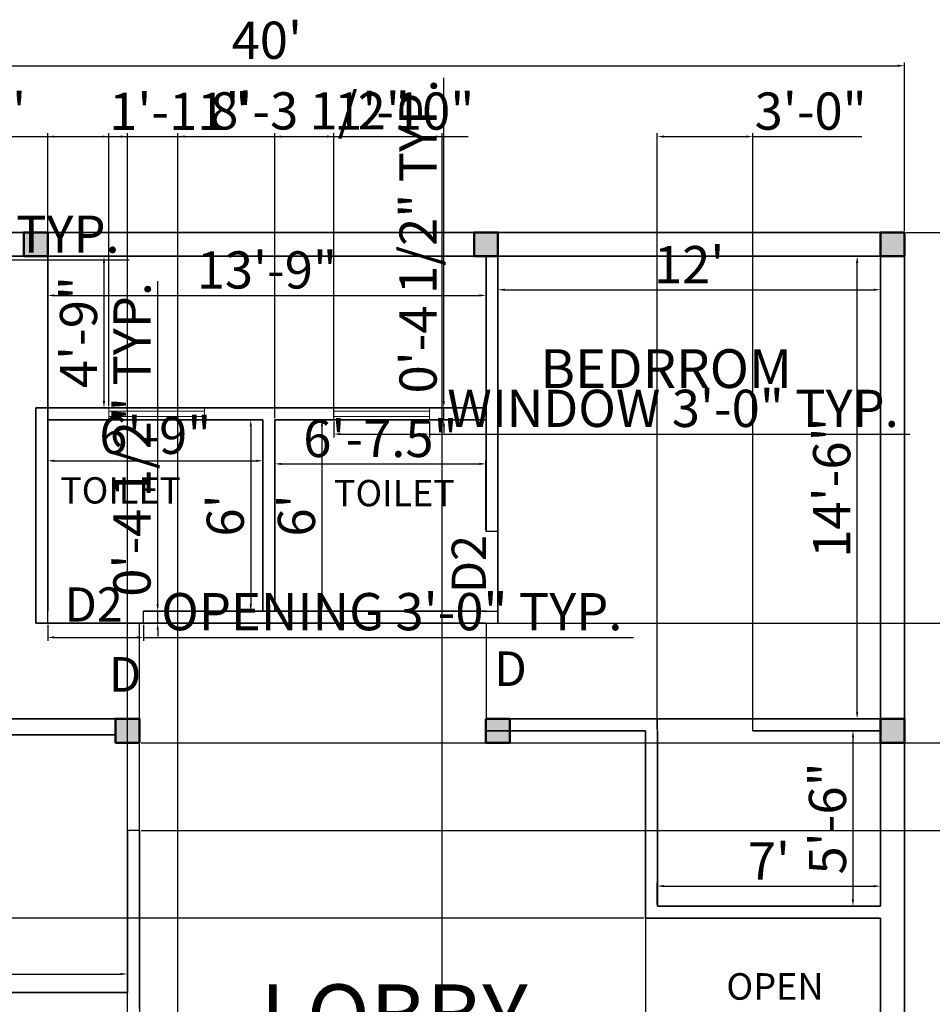
# Model space of a CAD drawing. Units: inches. Extents: x 3316 to 4157, y 2203 to 2977.
# Tile 3 of 4: x 3517 to 3860, y 2597 to 2968. Entities that reach past the tile are written whole.
import ezdxf

# ---------------------------------------------------------------- set-up
doc = ezdxf.new("R2010")
doc.units = ezdxf.units.IN
for name, color, linetype, lineweight in [('A-ANNO-DIMS', 2, 'Continuous', 18), ('A-ANNO-TEXT', 7, 'Continuous', 18), ('A-AREA-IDEN', 7, 'Continuous', 25), ('A-COLS', 7, 'Continuous', 50), ('A-COLS-PATT', 4, 'Continuous', 13), ('A-DOOR', 3, 'Continuous', 25), ('A-GLAZ', 4, 'Continuous', 18), ('A-WALL', 7, 'Continuous', 35), ('C-PROP', 7, 'Continuous', 35)]:
    doc.layers.add(name, color=color, linetype=linetype, lineweight=lineweight)
doc.styles.get("Standard").update_dxf_attribs({"font": 'arial.ttf'})
doc.dimstyles.new('ISO-25', dxfattribs={"dimtxt": 14, "dimasz": 2.5, "dimexe": 1.25, "dimexo": 0.625, "dimtad": 1, "dimlunit": 3, "dimtxsty": 'Standard', "dimcen": 2.5, "dimadec": 0, "dimazin": 0, "dimtfac": 1, "dimtmove": 0, "dimatfit": 3, "dimfxl": 1, "dimarcsym": 0})

# ---------------------------------------------------------------- blocks, each defined once
blk = doc.blocks.new('*D1')
at = {"layer": 'A-ANNO-DIMS', "color": 0, "lineweight": -2, "transparency": 16777216}
for p, q in [((3696.58, 2866.89), (3696.58, 2867.51)), ((3840.58, 2863.07), (3840.58, 2867.51)), ((3699.08, 2866.26), (3838.08, 2866.26))]:
    blk.add_line(p, q, dxfattribs=at)
at = {"layer": 'A-ANNO-DIMS', "color": 0, "transparency": 16777216}
for points in [[(3699.08, 2866.68), (3699.08, 2865.84), (3696.58, 2866.26)], [(3838.08, 2866.68), (3838.08, 2865.84), (3840.58, 2866.26)]]:
    blk.add_solid(points, dxfattribs=at)
at = {"layer": 'Defpoints', "color": 0, "transparency": 16777216}
for p in [(3696.58, 2866.26), (3840.58, 2866.26), (3840.58, 2862.44)]:
    blk.add_point(p, dxfattribs=at)
at = {"layer": 'A-ANNO-DIMS', "color": 0, "transparency": 16777216, "insert": (3768.58, 2873.91), "char_height": 14, "attachment_point": 5}
blk.add_mtext("12'", dxfattribs=at)
blk = doc.blocks.new('*D2')
at = {"layer": 'A-ANNO-DIMS', "color": 0, "lineweight": -2, "transparency": 16777216}
for p, q in [((3832.43, 2878.84), (3833.05, 2878.84)), ((3831.8, 2707.34), (3831.8, 2876.34)), ((3832.43, 2704.84), (3833.05, 2704.84))]:
    blk.add_line(p, q, dxfattribs=at)
at = {"layer": 'A-ANNO-DIMS', "color": 0, "transparency": 16777216}
for points in [[(3831.38, 2876.34), (3832.22, 2876.34), (3831.8, 2878.84)], [(3831.38, 2707.34), (3832.22, 2707.34), (3831.8, 2704.84)]]:
    blk.add_solid(points, dxfattribs=at)
at = {"layer": 'Defpoints', "color": 0, "transparency": 16777216}
for p in [(3831.8, 2878.84), (3831.8, 2878.84), (3831.8, 2704.84)]:
    blk.add_point(p, dxfattribs=at)
at = {"layer": 'A-ANNO-DIMS', "color": 0, "transparency": 16777216, "insert": (3824.03, 2791.84), "char_height": 14, "attachment_point": 5, "rotation": 90}
blk.add_mtext('14\'-6"', dxfattribs=at)
blk = doc.blocks.new('*D6')
at = {"layer": 'A-ANNO-DIMS', "color": 0, "lineweight": -2, "transparency": 16777216}
for p, q in [((3369.58, 2888.47), (3369.58, 2951.81)), ((3372.08, 2950.56), (3847.08, 2950.56)), ((3849.58, 2888.47), (3849.58, 2951.81))]:
    blk.add_line(p, q, dxfattribs=at)
at = {"layer": 'A-ANNO-DIMS', "color": 0, "transparency": 16777216}
for points in [[(3372.08, 2950.98), (3372.08, 2950.14), (3369.58, 2950.56)], [(3847.08, 2950.98), (3847.08, 2950.14), (3849.58, 2950.56)]]:
    blk.add_solid(points, dxfattribs=at)
at = {"layer": 'Defpoints', "color": 0, "transparency": 16777216}
for p in [(3849.58, 2950.56), (3369.58, 2887.84), (3849.58, 2887.84)]:
    blk.add_point(p, dxfattribs=at)
at = {"layer": 'A-ANNO-DIMS', "color": 0, "transparency": 16777216, "insert": (3609.58, 2958.33), "char_height": 14, "attachment_point": 5}
blk.add_mtext("40'", dxfattribs=at)
blk = doc.blocks.new('*D7')
at = {"layer": 'A-ANNO-DIMS', "color": 0, "lineweight": -2, "transparency": 16777216}
for p, q in [((3850.21, 2887.84), (4040.36, 2887.84)), ((4039.11, 2885.34), (4039.11, 2254.34)), ((3850.21, 2251.84), (4040.36, 2251.84))]:
    blk.add_line(p, q, dxfattribs=at)
at = {"layer": 'A-ANNO-DIMS', "color": 0, "transparency": 16777216}
for points in [[(4038.69, 2885.34), (4039.53, 2885.34), (4039.11, 2887.84)], [(4038.69, 2254.34), (4039.53, 2254.34), (4039.11, 2251.84)]]:
    blk.add_solid(points, dxfattribs=at)
at = {"layer": 'Defpoints', "color": 0, "transparency": 16777216}
for p in [(3849.58, 2887.84), (3849.58, 2251.84), (4039.11, 2251.84)]:
    blk.add_point(p, dxfattribs=at)
at = {"layer": 'A-ANNO-DIMS', "color": 0, "transparency": 16777216, "insert": (4031.33, 2569.84), "char_height": 14, "attachment_point": 5, "rotation": 90}
blk.add_mtext("53'", dxfattribs=at)
blk = doc.blocks.new('*D8')
at = {"layer": 'A-ANNO-DIMS', "color": 0, "lineweight": -2, "transparency": 16777216}
for p, q in [((3527.08, 2802.53), (3527.08, 2803.15)), ((3529.58, 2801.9), (3605.58, 2801.9)), ((3608.08, 2802.53), (3608.08, 2803.15))]:
    blk.add_line(p, q, dxfattribs=at)
at = {"layer": 'A-ANNO-DIMS', "color": 0, "transparency": 16777216}
for points in [[(3529.58, 2802.32), (3529.58, 2801.48), (3527.08, 2801.9)], [(3605.58, 2802.32), (3605.58, 2801.48), (3608.08, 2801.9)]]:
    blk.add_solid(points, dxfattribs=at)
at = {"layer": 'Defpoints', "color": 0, "transparency": 16777216}
for p in [(3527.08, 2801.9), (3608.08, 2801.9), (3608.08, 2801.9)]:
    blk.add_point(p, dxfattribs=at)
at = {"layer": 'A-ANNO-DIMS', "color": 0, "transparency": 16777216, "insert": (3567.58, 2809.67), "char_height": 14, "attachment_point": 5}
blk.add_mtext('6\'-9"', dxfattribs=at)
blk = doc.blocks.new('*D9')
at = {"layer": 'A-ANNO-DIMS', "color": 0, "lineweight": -2, "transparency": 16777216}
for p, q in [((3613.21, 2817.34), (3631.55, 2817.34)), ((3630.3, 2814.84), (3630.3, 2747.84)), ((3613.21, 2745.34), (3631.55, 2745.34))]:
    blk.add_line(p, q, dxfattribs=at)
at = {"layer": 'A-ANNO-DIMS', "color": 0, "transparency": 16777216}
for points in [[(3629.89, 2814.84), (3630.72, 2814.84), (3630.3, 2817.34)], [(3629.89, 2747.84), (3630.72, 2747.84), (3630.3, 2745.34)]]:
    blk.add_solid(points, dxfattribs=at)
at = {"layer": 'Defpoints', "color": 0, "transparency": 16777216}
for p in [(3612.58, 2817.34), (3612.58, 2745.34), (3630.3, 2745.34)]:
    blk.add_point(p, dxfattribs=at)
at = {"layer": 'A-ANNO-DIMS', "color": 0, "transparency": 16777216, "insert": (3622.53, 2781.34), "char_height": 14, "attachment_point": 5, "rotation": 90}
blk.add_mtext("6'", dxfattribs=at)
blk = doc.blocks.new('*D10')
at = {"layer": 'A-ANNO-DIMS', "color": 0, "lineweight": -2, "transparency": 16777216}
for p, q in [((3612.58, 2816.72), (3612.58, 2799.49)), ((3692.08, 2775.97), (3692.08, 2801.99)), ((3615.08, 2800.74), (3689.58, 2800.74))]:
    blk.add_line(p, q, dxfattribs=at)
at = {"layer": 'A-ANNO-DIMS', "color": 0, "transparency": 16777216}
for points in [[(3615.08, 2801.15), (3615.08, 2800.32), (3612.58, 2800.74)], [(3689.58, 2801.15), (3689.58, 2800.32), (3692.08, 2800.74)]]:
    blk.add_solid(points, dxfattribs=at)
at = {"layer": 'Defpoints', "color": 0, "transparency": 16777216}
for p in [(3612.58, 2817.34), (3692.08, 2800.74), (3692.08, 2775.34)]:
    blk.add_point(p, dxfattribs=at)
at = {"layer": 'A-ANNO-DIMS', "color": 0, "transparency": 16777216, "insert": (3652.33, 2808.51), "char_height": 14, "attachment_point": 5}
blk.add_mtext('6\'-7.5"', dxfattribs=at)
blk = doc.blocks.new('*D15')
at = {"layer": 'A-ANNO-DIMS', "color": 0, "lineweight": -2, "transparency": 16777216}
for p, q in [((3437.08, 2602.47), (3437.08, 2610.05)), ((3439.58, 2608.8), (3554.58, 2608.8)), ((3557.08, 2602.47), (3557.08, 2610.05))]:
    blk.add_line(p, q, dxfattribs=at)
at = {"layer": 'A-ANNO-DIMS', "color": 0, "transparency": 16777216}
for points in [[(3439.58, 2609.21), (3439.58, 2608.38), (3437.08, 2608.8)], [(3554.58, 2609.21), (3554.58, 2608.38), (3557.08, 2608.8)]]:
    blk.add_solid(points, dxfattribs=at)
at = {"layer": 'Defpoints', "color": 0, "transparency": 16777216}
for p in [(3557.08, 2608.8), (3437.08, 2601.84), (3557.08, 2601.84)]:
    blk.add_point(p, dxfattribs=at)
at = {"layer": 'A-ANNO-DIMS', "color": 0, "transparency": 16777216, "insert": (3497.08, 2616.57), "char_height": 14, "attachment_point": 5}
blk.add_mtext("10'", dxfattribs=at)
blk = doc.blocks.new('*D16')
at = {"layer": 'A-ANNO-DIMS', "color": 0, "lineweight": -2, "transparency": 16777216}
for p, q in [((3839.96, 2700.34), (3828.97, 2700.34)), ((3830.22, 2697.84), (3830.22, 2636.84)), ((3839.96, 2634.34), (3828.97, 2634.34))]:
    blk.add_line(p, q, dxfattribs=at)
at = {"layer": 'A-ANNO-DIMS', "color": 0, "transparency": 16777216}
for points in [[(3829.8, 2697.84), (3830.63, 2697.84), (3830.22, 2700.34)], [(3829.8, 2636.84), (3830.63, 2636.84), (3830.22, 2634.34)]]:
    blk.add_solid(points, dxfattribs=at)
at = {"layer": 'Defpoints', "color": 0, "transparency": 16777216}
for p in [(3840.58, 2700.34), (3830.22, 2634.34), (3840.58, 2634.34)]:
    blk.add_point(p, dxfattribs=at)
at = {"layer": 'A-ANNO-DIMS', "color": 0, "transparency": 16777216, "insert": (3822.44, 2667.34), "char_height": 14, "attachment_point": 5, "rotation": 90}
blk.add_mtext('5\'-6"', dxfattribs=at)
blk = doc.blocks.new('*D17')
at = {"layer": 'A-ANNO-DIMS', "color": 0, "lineweight": -2, "transparency": 16777216}
for p, q in [((3756.58, 2634.97), (3756.58, 2643.11)), ((3759.08, 2641.86), (3838.08, 2641.86)), ((3840.58, 2634.97), (3840.58, 2643.11))]:
    blk.add_line(p, q, dxfattribs=at)
at = {"layer": 'A-ANNO-DIMS', "color": 0, "transparency": 16777216}
for points in [[(3759.08, 2642.28), (3759.08, 2641.45), (3756.58, 2641.86)], [(3838.08, 2642.28), (3838.08, 2641.45), (3840.58, 2641.86)]]:
    blk.add_solid(points, dxfattribs=at)
at = {"layer": 'Defpoints', "color": 0, "transparency": 16777216}
for p in [(3840.58, 2641.86), (3756.58, 2634.34), (3840.58, 2634.34)]:
    blk.add_point(p, dxfattribs=at)
at = {"layer": 'A-ANNO-DIMS', "color": 0, "transparency": 16777216, "insert": (3798.58, 2649.49), "char_height": 14, "attachment_point": 5}
blk.add_mtext("7'", dxfattribs=at)
blk = doc.blocks.new('*D22')
at = {"layer": 'A-ANNO-DIMS', "color": 0, "lineweight": -2, "transparency": 16777216}
for p, q in [((3527.08, 2878.22), (3527.08, 2862.87)), ((3692.08, 2878.22), (3692.08, 2862.87)), ((3529.58, 2864.12), (3689.58, 2864.12))]:
    blk.add_line(p, q, dxfattribs=at)
at = {"layer": 'A-ANNO-DIMS', "color": 0, "transparency": 16777216}
for points in [[(3529.58, 2864.54), (3529.58, 2863.7), (3527.08, 2864.12)], [(3689.58, 2864.54), (3689.58, 2863.7), (3692.08, 2864.12)]]:
    blk.add_solid(points, dxfattribs=at)
at = {"layer": 'Defpoints', "color": 0, "transparency": 16777216}
for p in [(3527.08, 2878.84), (3692.08, 2878.84), (3692.08, 2864.12)]:
    blk.add_point(p, dxfattribs=at)
at = {"layer": 'A-ANNO-DIMS', "color": 0, "transparency": 16777216, "insert": (3609.58, 2871.9), "char_height": 14, "attachment_point": 5}
blk.add_mtext('13\'-9"', dxfattribs=at)
blk = doc.blocks.new('*D23')
at = {"layer": 'A-ANNO-DIMS', "color": 0, "lineweight": -2, "transparency": 16777216}
for p, q in [((3527.71, 2878.84), (3549.52, 2878.84)), ((3548.27, 2876.34), (3548.27, 2824.34)), ((3527.71, 2821.84), (3549.52, 2821.84))]:
    blk.add_line(p, q, dxfattribs=at)
at = {"layer": 'A-ANNO-DIMS', "color": 0, "transparency": 16777216}
for points in [[(3547.85, 2876.34), (3548.69, 2876.34), (3548.27, 2878.84)], [(3547.85, 2824.34), (3548.69, 2824.34), (3548.27, 2821.84)]]:
    blk.add_solid(points, dxfattribs=at)
at = {"layer": 'Defpoints', "color": 0, "transparency": 16777216}
for p in [(3527.08, 2878.84), (3527.08, 2821.84), (3548.27, 2821.84)]:
    blk.add_point(p, dxfattribs=at)
at = {"layer": 'A-ANNO-DIMS', "color": 0, "transparency": 16777216, "insert": (3540.5, 2850.34), "char_height": 14, "attachment_point": 5, "rotation": 90}
blk.add_mtext('4\'-9"', dxfattribs=at)
blk = doc.blocks.new('*D26')
at = {"layer": 'A-ANNO-DIMS', "color": 0, "lineweight": -2, "transparency": 16777216}
for p, q in [((3607.46, 2817.34), (3602.26, 2817.34)), ((3603.51, 2814.84), (3603.51, 2747.84)), ((3607.46, 2745.34), (3602.26, 2745.34))]:
    blk.add_line(p, q, dxfattribs=at)
at = {"layer": 'A-ANNO-DIMS', "color": 0, "transparency": 16777216}
for points in [[(3603.1, 2814.84), (3603.93, 2814.84), (3603.51, 2817.34)], [(3603.1, 2747.84), (3603.93, 2747.84), (3603.51, 2745.34)]]:
    blk.add_solid(points, dxfattribs=at)
at = {"layer": 'Defpoints', "color": 0, "transparency": 16777216}
for p in [(3608.08, 2817.34), (3603.51, 2745.34), (3608.08, 2745.34)]:
    blk.add_point(p, dxfattribs=at)
at = {"layer": 'A-ANNO-DIMS', "color": 0, "transparency": 16777216, "insert": (3595.74, 2781.34), "char_height": 14, "attachment_point": 5, "rotation": 90}
blk.add_mtext("6'", dxfattribs=at)
blk = doc.blocks.new('COL-9IN-SQ')
for p, q in [((0, 9), (0, 0)), ((9, 9), (0, 9)), ((9, 0), (9, 9)), ((0, 0), (9, 0))]:
    blk.add_line(p, q)
blk = doc.blocks.new('COL-9IN-SQ-PL')
blk.add_lwpolyline([(0, 0), (9, 0), (9, 9), (0, 9)], close=True)
blk = doc.blocks.new('WIN-36IN')
for p, q in [((0, 0), (0, 4.5)), ((36, 4.5), (36, 0)), ((0, 3.25), (36, 3.25)), ((0, 1.25), (36, 1.25)), ((36, 0), (0, 0))]:
    blk.add_line(p, q)
blk = doc.blocks.new('DOOR-36IN-OPENING')
for p, q in [((0, 0), (0, 4.5)), ((36, 0), (36, 4.5)), ((0, 0), (36, 0))]:
    blk.add_line(p, q)
blk = doc.blocks.new('DOOR-30IN-OPENING')
for p, q in [((4.5, 30), (0, 30)), ((4.5, 0), (4.5, 30)), ((0, 0), (4.5, 0))]:
    blk.add_line(p, q)
blk = doc.blocks.new('*D36')
at = {"layer": 'A-ANNO-DIMS', "color": 0, "lineweight": -2, "transparency": 16777216}
for p, q in [((3369.58, 2878.22), (3369.58, 2876.24)), ((3372.08, 2877.49), (3376.08, 2877.49)), ((3378.58, 2878.22), (3378.58, 2876.24)), ((3378.58, 2877.49), (3557.7, 2877.49))]:
    blk.add_line(p, q, dxfattribs=at)
at = {"layer": 'A-ANNO-DIMS', "color": 0, "transparency": 16777216}
for points in [[(3372.08, 2877.91), (3372.08, 2877.08), (3369.58, 2877.49)], [(3376.08, 2877.91), (3376.08, 2877.08), (3378.58, 2877.49)]]:
    blk.add_solid(points, dxfattribs=at)
at = {"layer": 'Defpoints', "color": 0, "transparency": 16777216}
for p in [(3369.58, 2878.84), (3378.58, 2878.84), (3378.58, 2877.49)]:
    blk.add_point(p, dxfattribs=at)
at = {"layer": 'A-ANNO-DIMS', "color": 0, "transparency": 16777216, "insert": (3469.39, 2885.36), "char_height": 14, "attachment_point": 5}
blk.add_mtext('COLUMN 0\'-9" TYP.', dxfattribs=at)
blk = doc.blocks.new('*D40')
at = {"layer": 'A-ANNO-DIMS', "color": 0, "lineweight": -2, "transparency": 16777216}
for p, q in [((3634.78, 2816.72), (3634.78, 2810.69)), ((3670.78, 2816.72), (3670.78, 2810.69)), ((3637.28, 2811.94), (3668.28, 2811.94)), ((3670.78, 2811.94), (3851.69, 2811.94))]:
    blk.add_line(p, q, dxfattribs=at)
at = {"layer": 'A-ANNO-DIMS', "color": 0, "transparency": 16777216}
for points in [[(3637.28, 2812.36), (3637.28, 2811.53), (3634.78, 2811.94)], [(3668.28, 2812.36), (3668.28, 2811.53), (3670.78, 2811.94)]]:
    blk.add_solid(points, dxfattribs=at)
at = {"layer": 'Defpoints', "color": 0, "transparency": 16777216}
for p in [(3634.78, 2817.34), (3670.78, 2817.34), (3670.78, 2811.94)]:
    blk.add_point(p, dxfattribs=at)
at = {"layer": 'A-ANNO-DIMS', "color": 0, "transparency": 16777216, "insert": (3762.48, 2819.82), "char_height": 14, "attachment_point": 5}
blk.add_mtext('WINDOW 3\'-0" TYP.', dxfattribs=at)
blk = doc.blocks.new('*D41')
at = {"layer": 'A-ANNO-DIMS', "color": 0, "lineweight": -2, "transparency": 16777216}
for p, q in [((3676.18, 2824.34), (3676.18, 2946.05)), ((3671.41, 2821.84), (3677.43, 2821.84)), ((3676.18, 2817.34), (3676.18, 2821.84)), ((3671.41, 2817.34), (3677.43, 2817.34)), ((3676.18, 2814.84), (3676.18, 2812.34))]:
    blk.add_line(p, q, dxfattribs=at)
at = {"layer": 'A-ANNO-DIMS', "color": 0, "transparency": 16777216}
for points in [[(3675.76, 2824.34), (3676.6, 2824.34), (3676.18, 2821.84)], [(3675.76, 2814.84), (3676.6, 2814.84), (3676.18, 2817.34)]]:
    blk.add_solid(points, dxfattribs=at)
at = {"layer": 'Defpoints', "color": 0, "transparency": 16777216}
for p in [(3670.78, 2821.84), (3676.18, 2821.84), (3670.78, 2817.34)]:
    blk.add_point(p, dxfattribs=at)
at = {"layer": 'A-ANNO-DIMS', "color": 0, "transparency": 16777216, "insert": (3668.32, 2886.45), "char_height": 14, "attachment_point": 5, "rotation": 90}
blk.add_mtext('0\'-4 1/2" TYP.', dxfattribs=at)
blk = doc.blocks.new('*D42')
at = {"layer": 'A-ANNO-DIMS', "color": 0, "lineweight": -2, "transparency": 16777216}
for p, q in [((3527.08, 2740.22), (3527.08, 2734.19)), ((3563.08, 2740.22), (3563.08, 2734.19)), ((3529.58, 2735.44), (3560.58, 2735.44)), ((3563.08, 2735.44), (3747.67, 2735.44))]:
    blk.add_line(p, q, dxfattribs=at)
at = {"layer": 'A-ANNO-DIMS', "color": 0, "transparency": 16777216}
for points in [[(3529.58, 2735.86), (3529.58, 2735.03), (3527.08, 2735.44)], [(3560.58, 2735.86), (3560.58, 2735.03), (3563.08, 2735.44)]]:
    blk.add_solid(points, dxfattribs=at)
at = {"layer": 'Defpoints', "color": 0, "transparency": 16777216}
for p in [(3527.08, 2740.84), (3563.08, 2740.84), (3563.08, 2735.44)]:
    blk.add_point(p, dxfattribs=at)
at = {"layer": 'A-ANNO-DIMS', "color": 0, "transparency": 16777216, "insert": (3656.63, 2743.32), "char_height": 14, "attachment_point": 5}
blk.add_mtext('OPENING 3\'-0" TYP.', dxfattribs=at)
blk = doc.blocks.new('*D43')
at = {"layer": 'A-ANNO-DIMS', "color": 0, "lineweight": -2, "transparency": 16777216}
for p, q in [((3568.48, 2747.84), (3568.48, 2869.55)), ((3563.71, 2745.34), (3569.73, 2745.34)), ((3568.48, 2740.84), (3568.48, 2745.34)), ((3563.71, 2740.84), (3569.73, 2740.84)), ((3568.48, 2738.34), (3568.48, 2735.84))]:
    blk.add_line(p, q, dxfattribs=at)
at = {"layer": 'A-ANNO-DIMS', "color": 0, "transparency": 16777216}
for points in [[(3568.07, 2747.84), (3568.9, 2747.84), (3568.48, 2745.34)], [(3568.07, 2738.34), (3568.9, 2738.34), (3568.48, 2740.84)]]:
    blk.add_solid(points, dxfattribs=at)
at = {"layer": 'Defpoints', "color": 0, "transparency": 16777216}
for p in [(3563.08, 2745.34), (3568.48, 2745.34), (3563.08, 2740.84)]:
    blk.add_point(p, dxfattribs=at)
at = {"layer": 'A-ANNO-DIMS', "color": 0, "transparency": 16777216, "insert": (3560.62, 2809.95), "char_height": 14, "attachment_point": 5, "rotation": 90}
blk.add_mtext('0\'-4 1/2" TYP.', dxfattribs=at)
blk = doc.blocks.new('*D48')
at = {"layer": 'A-ANNO-DIMS', "color": 0, "lineweight": -2, "transparency": 16777216}
for p, q in [((3527.08, 2822.47), (3527.08, 2925.14)), ((3529.58, 2923.89), (3547.61, 2923.89)), ((3550.11, 2822.47), (3550.11, 2925.14)), ((3550.11, 2923.89), (3600.63, 2923.89))]:
    blk.add_line(p, q, dxfattribs=at)
at = {"layer": 'A-ANNO-DIMS', "color": 0, "transparency": 16777216}
for points in [[(3529.58, 2924.31), (3529.58, 2923.48), (3527.08, 2923.89)], [(3547.61, 2924.31), (3547.61, 2923.48), (3550.11, 2923.89)]]:
    blk.add_solid(points, dxfattribs=at)
at = {"layer": 'Defpoints', "color": 0, "transparency": 16777216}
for p in [(3550.11, 2923.89), (3527.08, 2821.84), (3550.11, 2821.84)]:
    blk.add_point(p, dxfattribs=at)
at = {"layer": 'A-ANNO-DIMS', "color": 0, "transparency": 16777216, "insert": (3576.62, 2931.55), "char_height": 14, "attachment_point": 5}
blk.add_mtext('1\'-11"', dxfattribs=at)
blk = doc.blocks.new('*D49')
at = {"layer": 'A-ANNO-DIMS', "color": 0, "lineweight": -2, "transparency": 16777216}
for p, q in [((3612.58, 2817.97), (3612.58, 2925.14)), ((3615.08, 2923.89), (3632.28, 2923.89)), ((3634.78, 2817.97), (3634.78, 2925.14)), ((3634.78, 2923.89), (3685.31, 2923.89))]:
    blk.add_line(p, q, dxfattribs=at)
at = {"layer": 'A-ANNO-DIMS', "color": 0, "transparency": 16777216}
for points in [[(3615.08, 2924.31), (3615.08, 2923.48), (3612.58, 2923.89)], [(3632.28, 2924.31), (3632.28, 2923.48), (3634.78, 2923.89)]]:
    blk.add_solid(points, dxfattribs=at)
at = {"layer": 'Defpoints', "color": 0, "transparency": 16777216}
for p in [(3634.78, 2923.89), (3612.58, 2817.34), (3634.78, 2817.34)]:
    blk.add_point(p, dxfattribs=at)
at = {"layer": 'A-ANNO-DIMS', "color": 0, "transparency": 16777216, "insert": (3661.29, 2931.67), "char_height": 14, "attachment_point": 5}
blk.add_mtext('1\'-10"', dxfattribs=at)
blk = doc.blocks.new('*D50')
at = {"layer": 'A-ANNO-DIMS', "color": 0, "lineweight": -2, "transparency": 16777216}
for p, q in [((3751.46, 2629.84), (3332.28, 2629.84)), ((3333.53, 2627.34), (3333.53, 2578.34)), ((3751.46, 2575.84), (3332.28, 2575.84))]:
    blk.add_line(p, q, dxfattribs=at)
at = {"layer": 'A-ANNO-DIMS', "color": 0, "transparency": 16777216}
for points in [[(3333.12, 2627.34), (3333.95, 2627.34), (3333.53, 2629.84)], [(3333.12, 2578.34), (3333.95, 2578.34), (3333.53, 2575.84)]]:
    blk.add_solid(points, dxfattribs=at)
at = {"layer": 'Defpoints', "color": 0, "transparency": 16777216}
for p in [(3752.08, 2629.84), (3333.53, 2575.84), (3752.08, 2575.84)]:
    blk.add_point(p, dxfattribs=at)
at = {"layer": 'A-ANNO-DIMS', "color": 0, "transparency": 16777216, "insert": (3325.76, 2602.84), "char_height": 14, "attachment_point": 5, "rotation": 90}
blk.add_mtext('4\'-6"', dxfattribs=at)
blk = doc.blocks.new('*D51')
at = {"layer": 'A-ANNO-DIMS', "color": 0, "lineweight": -2, "transparency": 16777216}
for p, q in [((3562.21, 2695.84), (3886.88, 2695.84)), ((3885.63, 2693.34), (3885.63, 2665.34)), ((3562.21, 2662.84), (3886.88, 2662.84)), ((3885.63, 2662.84), (3885.63, 2621.64))]:
    blk.add_line(p, q, dxfattribs=at)
at = {"layer": 'A-ANNO-DIMS', "color": 0, "transparency": 16777216}
for points in [[(3885.22, 2693.34), (3886.05, 2693.34), (3885.63, 2695.84)], [(3885.22, 2665.34), (3886.05, 2665.34), (3885.63, 2662.84)]]:
    blk.add_solid(points, dxfattribs=at)
at = {"layer": 'Defpoints', "color": 0, "transparency": 16777216}
for p in [(3561.58, 2695.84), (3561.58, 2662.84), (3885.63, 2662.84)]:
    blk.add_point(p, dxfattribs=at)
at = {"layer": 'A-ANNO-DIMS', "color": 0, "transparency": 16777216, "insert": (3877.86, 2640.99), "char_height": 14, "attachment_point": 5, "rotation": 90}
blk.add_mtext('2\'-9"', dxfattribs=at)
blk = doc.blocks.new('*D52')
at = {"layer": 'A-ANNO-DIMS', "color": 0, "lineweight": -2, "transparency": 16777216}
for p, q in [((3576.12, 2505.97), (3576.12, 2925.14)), ((3578.62, 2923.89), (3673.07, 2923.89)), ((3675.57, 2505.97), (3675.57, 2925.14))]:
    blk.add_line(p, q, dxfattribs=at)
at = {"layer": 'A-ANNO-DIMS', "color": 0, "transparency": 16777216}
for points in [[(3578.62, 2924.31), (3578.62, 2923.48), (3576.12, 2923.89)], [(3673.07, 2924.31), (3673.07, 2923.48), (3675.57, 2923.89)]]:
    blk.add_solid(points, dxfattribs=at)
at = {"layer": 'Defpoints', "color": 0, "transparency": 16777216}
for p in [(3675.57, 2923.89), (3576.12, 2505.34), (3675.57, 2505.34)]:
    blk.add_point(p, dxfattribs=at)
at = {"layer": 'A-ANNO-DIMS', "color": 0, "transparency": 16777216, "insert": (3625.84, 2931.76), "char_height": 14, "attachment_point": 5}
blk.add_mtext('8\'-3 1/2"', dxfattribs=at)
blk = doc.blocks.new('*D56')
at = {"layer": 'A-ANNO-DIMS', "color": 0, "lineweight": -2, "transparency": 16777216}
for p, q in [((3752.08, 2699.72), (3752.08, 2214.54)), ((3561.58, 2662.22), (3561.58, 2214.54)), ((3564.08, 2215.79), (3749.58, 2215.79))]:
    blk.add_line(p, q, dxfattribs=at)
at = {"layer": 'A-ANNO-DIMS', "color": 0, "transparency": 16777216}
for points in [[(3564.08, 2216.21), (3564.08, 2215.38), (3561.58, 2215.79)], [(3749.58, 2216.21), (3749.58, 2215.38), (3752.08, 2215.79)]]:
    blk.add_solid(points, dxfattribs=at)
at = {"layer": 'Defpoints', "color": 0, "transparency": 16777216}
for p in [(3752.08, 2700.34), (3561.58, 2662.84), (3752.08, 2215.79)]:
    blk.add_point(p, dxfattribs=at)
at = {"layer": 'A-ANNO-DIMS', "color": 0, "transparency": 16777216, "insert": (3656.83, 2223.66), "char_height": 14, "attachment_point": 5}
blk.add_mtext('15\'-10 1/2"', dxfattribs=at)
blk = doc.blocks.new('*D57')
at = {"layer": 'A-ANNO-DIMS', "color": 0, "lineweight": -2, "transparency": 16777216}
for p, q in [((3692.71, 2740.84), (3886.88, 2740.84)), ((3885.63, 2507.84), (3885.63, 2738.34)), ((3676.19, 2505.34), (3886.88, 2505.34))]:
    blk.add_line(p, q, dxfattribs=at)
at = {"layer": 'A-ANNO-DIMS', "color": 0, "transparency": 16777216}
for points in [[(3885.22, 2738.34), (3886.05, 2738.34), (3885.63, 2740.84)], [(3885.22, 2507.84), (3886.05, 2507.84), (3885.63, 2505.34)]]:
    blk.add_solid(points, dxfattribs=at)
at = {"layer": 'Defpoints', "color": 0, "transparency": 16777216}
for p in [(3692.08, 2740.84), (3885.63, 2740.84), (3675.57, 2505.34)]:
    blk.add_point(p, dxfattribs=at)
at = {"layer": 'A-ANNO-DIMS', "color": 0, "transparency": 16777216, "insert": (3877.77, 2623.09), "char_height": 14, "attachment_point": 5, "rotation": 90}
blk.add_mtext('19\'-7 1/2"', dxfattribs=at)
blk = doc.blocks.new('*D58')
at = {"layer": 'A-ANNO-DIMS', "color": 0, "lineweight": -2, "transparency": 16777216}
for p, q in [((3756.58, 2700.97), (3756.58, 2925.14)), ((3759.08, 2923.89), (3790.08, 2923.89)), ((3792.58, 2700.97), (3792.58, 2925.14)), ((3792.58, 2923.89), (3833.54, 2923.89))]:
    blk.add_line(p, q, dxfattribs=at)
at = {"layer": 'A-ANNO-DIMS', "color": 0, "transparency": 16777216}
for points in [[(3759.08, 2924.31), (3759.08, 2923.48), (3756.58, 2923.89)], [(3790.08, 2924.31), (3790.08, 2923.48), (3792.58, 2923.89)]]:
    blk.add_solid(points, dxfattribs=at)
at = {"layer": 'Defpoints', "color": 0, "transparency": 16777216}
for p in [(3792.58, 2923.89), (3756.58, 2700.34), (3792.58, 2700.34)]:
    blk.add_point(p, dxfattribs=at)
at = {"layer": 'A-ANNO-DIMS', "color": 0, "transparency": 16777216, "insert": (3814.31, 2931.67), "char_height": 14, "attachment_point": 5}
blk.add_mtext('3\'-0"', dxfattribs=at)
blk = doc.blocks.new('*D60')
at = {"layer": 'A-ANNO-DIMS', "color": 0, "lineweight": -2, "transparency": 16777216}
for p, q in [((3428.08, 2544.97), (3428.08, 2925.14)), ((3430.58, 2923.89), (3554.58, 2923.89)), ((3557.08, 2544.97), (3557.08, 2925.14))]:
    blk.add_line(p, q, dxfattribs=at)
at = {"layer": 'A-ANNO-DIMS', "color": 0, "transparency": 16777216}
for points in [[(3430.58, 2924.31), (3430.58, 2923.48), (3428.08, 2923.89)], [(3554.58, 2924.31), (3554.58, 2923.48), (3557.08, 2923.89)]]:
    blk.add_solid(points, dxfattribs=at)
at = {"layer": 'Defpoints', "color": 0, "transparency": 16777216}
for p in [(3557.08, 2923.89), (3428.08, 2544.34), (3557.08, 2544.34)]:
    blk.add_point(p, dxfattribs=at)
at = {"layer": 'A-ANNO-DIMS', "color": 0, "transparency": 16777216, "insert": (3492.58, 2931.67), "char_height": 14, "attachment_point": 5}
blk.add_mtext('10\'-9"', dxfattribs=at)

msp = doc.modelspace()

# ---------------------------------------------------------------- hatches: boundary and pattern name
at = {"layer": 'A-COLS-PATT'}
h = msp.add_hatch(color=256, dxfattribs=at)
h.dxf.hatch_style = 1
h.paths.add_polyline_path([(3849.584, 2887.842), (3840.584, 2887.842), (3840.584, 2878.842), (3849.584, 2878.842)])
h.paths.add_polyline_path([(3696.584, 2887.842), (3687.584, 2887.842), (3687.584, 2878.842), (3696.584, 2878.842)])
h.paths.add_polyline_path([(3527.084, 2887.842), (3518.084, 2887.842), (3518.084, 2878.842), (3527.084, 2878.842)])
h.paths.add_polyline_path([(3378.584, 2887.842), (3369.584, 2887.842), (3369.584, 2878.842), (3378.584, 2878.842)])
h.paths.add_polyline_path([(3378.584, 2707.842), (3369.584, 2707.842), (3369.584, 2698.842), (3378.584, 2698.842)])
h.paths.add_polyline_path([(3561.584, 2704.842), (3552.584, 2704.842), (3552.584, 2695.842), (3561.584, 2695.842)])
h.paths.add_polyline_path([(3701.03, 2704.842), (3692.084, 2704.842), (3692.084, 2700.342), (3701.03, 2700.342)])
h.paths.add_polyline_path([(3701.03, 2700.342), (3692.03, 2700.342), (3692.03, 2695.842), (3701.03, 2695.842)])
h.paths.add_polyline_path([(3849.584, 2704.835), (3840.584, 2704.835), (3840.584, 2695.835), (3849.584, 2695.835)])
h.paths.add_polyline_path([(3378.584, 2505.342), (3369.584, 2505.342), (3369.584, 2496.342), (3378.584, 2496.342)])
h.paths.add_polyline_path([(3378.584, 2357.104), (3369.584, 2357.104), (3369.584, 2348.104), (3378.584, 2348.104)])
h.paths.add_polyline_path([(3512.084, 2505.342), (3503.084, 2505.342), (3503.084, 2496.342), (3512.084, 2496.342)])
h.paths.add_polyline_path([(3512.084, 2356.842), (3503.084, 2356.842), (3503.084, 2347.842), (3512.084, 2347.842)])
h.paths.add_polyline_path([(3701.115, 2505.342), (3696.584, 2505.342), (3696.584, 2500.842), (3696.584, 2496.342), (3701.115, 2496.342)])
h.paths.add_polyline_path([(3696.584, 2505.342), (3692.115, 2505.342), (3692.115, 2496.342), (3696.584, 2496.342), (3696.584, 2500.842)])
h.paths.add_polyline_path([(3699.422, 2356.842), (3690.422, 2356.842), (3690.422, 2347.842), (3699.422, 2347.842)])
h.paths.add_polyline_path([(3849.584, 2356.899), (3840.584, 2356.899), (3840.584, 2347.899), (3849.584, 2347.899)])
h.paths.add_polyline_path([(3849.584, 2505.307), (3840.584, 2505.307), (3840.584, 2496.307), (3849.584, 2496.307)])

# ---------------------------------------------------------------- linework, layer by layer
at = {"layer": 'A-DOOR'}
for p, q in [((3561.584, 2662.842), (3561.584, 2740.842)), ((3561.584, 2698.842), (3561.584, 2704.842)), ((3756.584, 2700.342), (3756.584, 2704.842)), ((3792.584, 2700.342), (3792.584, 2704.842)), ((3561.584, 2662.842), (3557.084, 2662.842))]:
    msp.add_line(p, q, dxfattribs=at)
at = {"layer": 'A-GLAZ'}
msp.add_line((3582.113, 2817.342), (3546.113, 2817.342), dxfattribs=at)
at = {"layer": 'A-WALL'}
for p, q in [((3527.084, 2817.342), (3527.084, 2878.842)), ((3692.084, 2775.342), (3692.084, 2878.842)), ((3696.584, 2745.342), (3696.584, 2878.842)), ((3840.584, 2878.842), (3840.584, 2704.842)), ((3522.584, 2740.842), (3522.584, 2821.842)), ((3527.084, 2821.842), (3522.584, 2821.842)), ((3692.084, 2821.842), (3527.084, 2821.842)), ((3692.084, 2817.342), (3692.084, 2821.842)), ((3527.084, 2745.342), (3527.084, 2817.342)), ((3527.084, 2817.342), (3608.084, 2817.342)), ((3608.084, 2817.342), (3608.084, 2745.342)), ((3612.584, 2745.342), (3612.584, 2817.342)), ((3612.584, 2817.342), (3692.084, 2817.342)), ((3692.084, 2745.342), (3563.084, 2745.342)), ((3608.084, 2745.342), (3612.584, 2745.342)), ((3696.584, 2745.342), (3696.584, 2740.842)), ((3527.084, 2740.842), (3522.584, 2740.842)), ((3692.084, 2740.842), (3527.084, 2740.842)), ((3378.584, 2704.842), (3561.584, 2704.842)), ((3692.084, 2704.842), (3692.084, 2700.342)), ((3840.584, 2704.842), (3696.584, 2704.842)), ((3437.084, 2698.842), (3552.584, 2698.842)), ((3752.084, 2700.342), (3692.084, 2700.342)), ((3752.084, 2629.842), (3752.084, 2700.342)), ((3756.584, 2634.342), (3756.584, 2700.342)), ((3840.584, 2700.342), (3792.584, 2700.342)), ((3840.584, 2700.342), (3840.584, 2634.342)), ((3557.084, 2662.842), (3557.084, 2601.842)), ((3561.584, 2595.842), (3561.584, 2662.842)), ((3840.584, 2634.342), (3756.584, 2634.342)), ((3840.584, 2629.842), (3752.084, 2629.842)), ((3840.584, 2629.842), (3840.584, 2575.842)), ((3557.084, 2601.842), (3437.084, 2601.842))]:
    msp.add_line(p, q, dxfattribs=at)
for points in [[(3840.584, 2704.842), (3840.584, 2878.842), (3378.584, 2878.842), (3378.584, 2704.842)], [(3840.584, 2634.342), (3840.584, 2700.342)], [(3840.584, 2575.842), (3840.584, 2629.842)]]:
    msp.add_lwpolyline(points, dxfattribs=at)
at = {"layer": 'C-PROP'}
msp.add_lwpolyline([(3369.584, 2251.842), (3849.584, 2251.842), (3849.584, 2887.842), (3369.584, 2887.842)], close=True, dxfattribs=at)

# ---------------------------------------------------------------- block references
at = {"layer": 'A-COLS'}
for name, p in [('COL-9IN-SQ-PL', (3518.084, 2878.842)), ('COL-9IN-SQ-PL', (3687.584, 2878.842)), ('COL-9IN-SQ-PL', (3840.584, 2878.842)), ('COL-9IN-SQ-PL', (3552.584, 2695.842)), ('COL-9IN-SQ', (3692.031, 2695.842)), ('COL-9IN-SQ', (3840.584, 2695.836))]:
    msp.add_blockref(name, p, dxfattribs=at)
at = {"layer": 'A-DOOR'}
for name, p in [('DOOR-30IN-OPENING', (3692.084, 2745.342)), ('DOOR-36IN-OPENING', (3527.084, 2740.842))]:
    msp.add_blockref(name, p, dxfattribs=at)
at = {"layer": 'A-DOOR', "rotation": 270.0000000000014}
msp.add_blockref('DOOR-36IN-OPENING', (3692.084, 2740.842), dxfattribs=at)
at = {"layer": 'A-GLAZ'}
for p in [(3550.107, 2817.342), (3634.781, 2817.342)]:
    msp.add_blockref('WIN-36IN', p, dxfattribs=at)

# ---------------------------------------------------------------- texts
at = {"layer": 'A-ANNO-TEXT', "insert": (3679.158, 2752.139), "char_height": 12.8733, "attachment_point": 1, "rotation": 90}
msp.add_mtext_dynamic_manual_height_columns('D2', width=0.87177, gutter_width=64.367, heights=[0], dxfattribs=at)
at = {"layer": 'A-ANNO-TEXT', "attachment_point": 1}
for s, width, gutter_width, insert, char_height in [('D2', 0.87177, 64.367, (3533.494, 2754.275), 12.8733), ('D', 18.0935, 65.127, (3550.074, 2728.035), 13.025), ('D', 18.0935, 65.127, (3695.222, 2730.175), 13.025)]:
    msp.add_mtext_dynamic_manual_height_columns(s, width=width, gutter_width=gutter_width, heights=[0], dxfattribs=dict(at, insert=insert, char_height=char_height))
at = {"layer": 'A-AREA-IDEN', "attachment_point": 1}
for s, width, gutter_width, heights, insert, char_height in [('BEDRROM', 223.84192, 72.961, [0], (3712.52, 2843.883), 14.5923), ('TOILET', 14.33724, 49.489, [0], (3531.793, 2795.72), 9.8977), ('TOILET', 14.33724, 49.489, [0], (3634.87, 2794.692), 9.8977), ('OPEN', 86.57889, 49.928, [10.333], (3782.573, 2609.114), 9.9856)]:
    msp.add_mtext_dynamic_manual_height_columns(s, width=width, gutter_width=gutter_width, heights=heights, dxfattribs=dict(at, insert=insert, char_height=char_height))
at = {"layer": 'A-AREA-IDEN', "insert": (3607.117, 2604.899), "char_height": 23.5794, "attachment_point": 1}
msp.add_mtext('LOBBY', dxfattribs=at)

# ---------------------------------------------------------------- dimensions: what is measured, and where the dimension line sits
at = {"layer": 'A-ANNO-DIMS'}
for base, p1, p2, override, picture, middle in [((3849.584, 2950.561), (3369.584, 2887.842), (3849.584, 2887.842), {"dimclrd": 0, "dimclre": 0, "dimclrt": 0}, '*D6', (3609.584, 2958.334)), ((3675.569, 2923.892), (3576.116, 2505.342), (3675.569, 2505.342), {"dimdec": 1, "dimlfac": 1, "dimrnd": 0, "dimzin": 1, "dimdsep": 46, "dimlunit": 4, "dimfrac": 2}, '*D52', (3625.843, 2931.761)), ((3557.084, 2923.892), (3428.084, 2544.342), (3557.084, 2544.342), {"dimdec": 1, "dimlfac": 1, "dimrnd": 0, "dimzin": 1, "dimdsep": 46, "dimlunit": 4, "dimfrac": 2}, '*D60', (3492.584, 2931.665)), ((3550.107, 2923.892), (3527.084, 2821.842), (3550.107, 2821.842), {"dimdec": 1, "dimlfac": 1, "dimrnd": 0, "dimzin": 1, "dimdsep": 46, "dimlunit": 4, "dimfrac": 2}, '*D48', (3576.619, 2931.546)), ((3634.781, 2923.892), (3612.584, 2817.342), (3634.781, 2817.342), {"dimdec": 1, "dimlfac": 1, "dimrnd": 0, "dimzin": 1, "dimdsep": 46, "dimlunit": 4, "dimfrac": 2}, '*D49', (3661.293, 2931.665)), ((3792.584, 2923.892), (3756.584, 2700.342), (3792.584, 2700.342), {"dimdec": 1, "dimlfac": 1, "dimrnd": 0, "dimzin": 1, "dimdsep": 46, "dimlunit": 4, "dimfrac": 2}, '*D58', (3814.312, 2931.67)), ((3692.084, 2864.12), (3527.084, 2878.842), (3692.084, 2878.842), {"dimclrd": 0, "dimclre": 0, "dimclrt": 0}, '*D22', (3609.584, 2871.898)), ((3692.084, 2800.736), (3612.584, 2817.342), (3692.084, 2775.342), {"dimclrd": 0, "dimclre": 0, "dimclrt": 0}, '*D10', (3652.334, 2808.509)), ((3752.084, 2215.792), (3561.584, 2662.842), (3752.084, 2700.342), {"dimdec": 1, "dimlfac": 1, "dimrnd": 0, "dimzin": 1, "dimdsep": 46, "dimlunit": 4, "dimfrac": 2}, '*D56', (3656.834, 2223.656)), ((3840.584, 2641.865), (3756.584, 2634.342), (3840.584, 2634.342), {"dimclrd": 0, "dimclre": 0, "dimclrt": 0}, '*D17', (3798.584, 2649.49)), ((3557.084, 2608.797), (3437.084, 2601.842), (3557.084, 2601.842), {"dimclrd": 0, "dimclre": 0, "dimclrt": 0}, '*D15', (3497.084, 2616.57))]:
    dim = msp.add_linear_dim(base=base, p1=p1, p2=p2, dimstyle='ISO-25', override=override, dxfattribs=at)
    dim.commit()
    dim.dimension.update_dxf_attribs({"geometry": picture, "text_midpoint": middle})
for base, p1, p2, picture, middle in [((3676.181, 2821.842), (3670.781, 2817.342), (3670.781, 2821.842), '*D41', (3668.317, 2886.447)), ((3568.484, 2745.342), (3563.084, 2740.842), (3563.084, 2745.342), '*D43', (3560.62, 2809.947))]:
    dim = msp.add_linear_dim(base=base, p1=p1, p2=p2, angle=90, text='<> TYP.', dimstyle='ISO-25', override={"dimdec": 1, "dimlfac": 1, "dimrnd": 0, "dimzin": 1, "dimdsep": 46, "dimlunit": 4, "dimfrac": 2}, dxfattribs=at)
    dim.commit()
    dim.dimension.update_dxf_attribs({"geometry": picture, "text_midpoint": middle})
for base, p1, p2, text, picture, middle in [((3378.584, 2877.492), (3369.584, 2878.842), (3378.584, 2878.842), 'COLUMN <> TYP.', '*D36', (3469.39, 2885.361)), ((3670.781, 2811.942), (3634.781, 2817.342), (3670.781, 2817.342), 'WINDOW <> TYP.', '*D40', (3762.485, 2819.815)), ((3563.084, 2735.442), (3527.084, 2740.842), (3563.084, 2740.842), 'OPENING <> TYP.', '*D42', (3656.626, 2743.315))]:
    dim = msp.add_linear_dim(base=base, p1=p1, p2=p2, text=text, dimstyle='ISO-25', override={"dimdec": 1, "dimlfac": 1, "dimrnd": 0, "dimzin": 1, "dimdsep": 46, "dimlunit": 4, "dimfrac": 2}, dxfattribs=at)
    dim.commit()
    dim.dimension.update_dxf_attribs({"geometry": picture, "text_midpoint": middle})
for base, p1, p2, angle, override, picture, middle in [((4039.111, 2251.842), (3849.584, 2887.842), (3849.584, 2251.842), 90, {"dimclrd": 0, "dimclre": 0, "dimclrt": 0}, '*D7', (4031.333, 2569.842)), ((3840.584, 2866.26), (3696.584, 2866.26), (3840.584, 2862.443), 180, {"dimclrd": 0, "dimclre": 0, "dimclrt": 0}, '*D1', (3768.584, 2873.914)), ((3548.271, 2821.842), (3527.084, 2878.842), (3527.084, 2821.842), 90, {"dimclrd": 0, "dimclre": 0, "dimclrt": 0}, '*D23', (3540.498, 2850.342)), ((3831.801, 2878.842), (3831.801, 2704.842), (3831.801, 2878.842), 270, {"dimclrd": 0, "dimclre": 0, "dimclrt": 0}, '*D2', (3824.028, 2791.842)), ((3608.084, 2801.902), (3527.084, 2801.902), (3608.084, 2801.902), 180, {"dimclrd": 0, "dimclre": 0, "dimclrt": 0}, '*D8', (3567.584, 2809.675)), ((3603.515, 2745.342), (3608.084, 2817.342), (3608.084, 2745.342), 90, {"dimclrd": 0, "dimclre": 0, "dimclrt": 0}, '*D26', (3595.742, 2781.342)), ((3630.303, 2745.342), (3612.584, 2817.342), (3612.584, 2745.342), 90, {"dimclrd": 0, "dimclre": 0, "dimclrt": 0}, '*D9', (3622.53, 2781.342)), ((3885.634, 2740.842), (3675.569, 2505.342), (3692.084, 2740.842), 90, {"dimdec": 1, "dimlfac": 1, "dimrnd": 0, "dimzin": 1, "dimdsep": 46, "dimlunit": 4, "dimfrac": 2}, '*D57', (3877.77, 2623.092)), ((3830.216, 2634.342), (3840.584, 2700.342), (3840.584, 2634.342), 90, {"dimclrd": 0, "dimclre": 0, "dimclrt": 0}, '*D16', (3822.443, 2667.342)), ((3885.634, 2662.842), (3561.584, 2695.842), (3561.584, 2662.842), 90, {"dimdec": 1, "dimlfac": 1, "dimrnd": 0, "dimzin": 1, "dimdsep": 46, "dimlunit": 4, "dimfrac": 2}, '*D51', (3877.861, 2640.99)), ((3333.534, 2575.842), (3752.084, 2629.842), (3752.084, 2575.842), 90, {"dimdec": 1, "dimlfac": 1, "dimrnd": 0, "dimzin": 1, "dimdsep": 46, "dimlunit": 4, "dimfrac": 2}, '*D50', (3325.761, 2602.842))]:
    dim = msp.add_linear_dim(base=base, p1=p1, p2=p2, angle=angle, dimstyle='ISO-25', override=override, dxfattribs=at)
    dim.commit()
    dim.dimension.update_dxf_attribs({"geometry": picture, "text_midpoint": middle})

doc.saveas('drawing.dxf')
